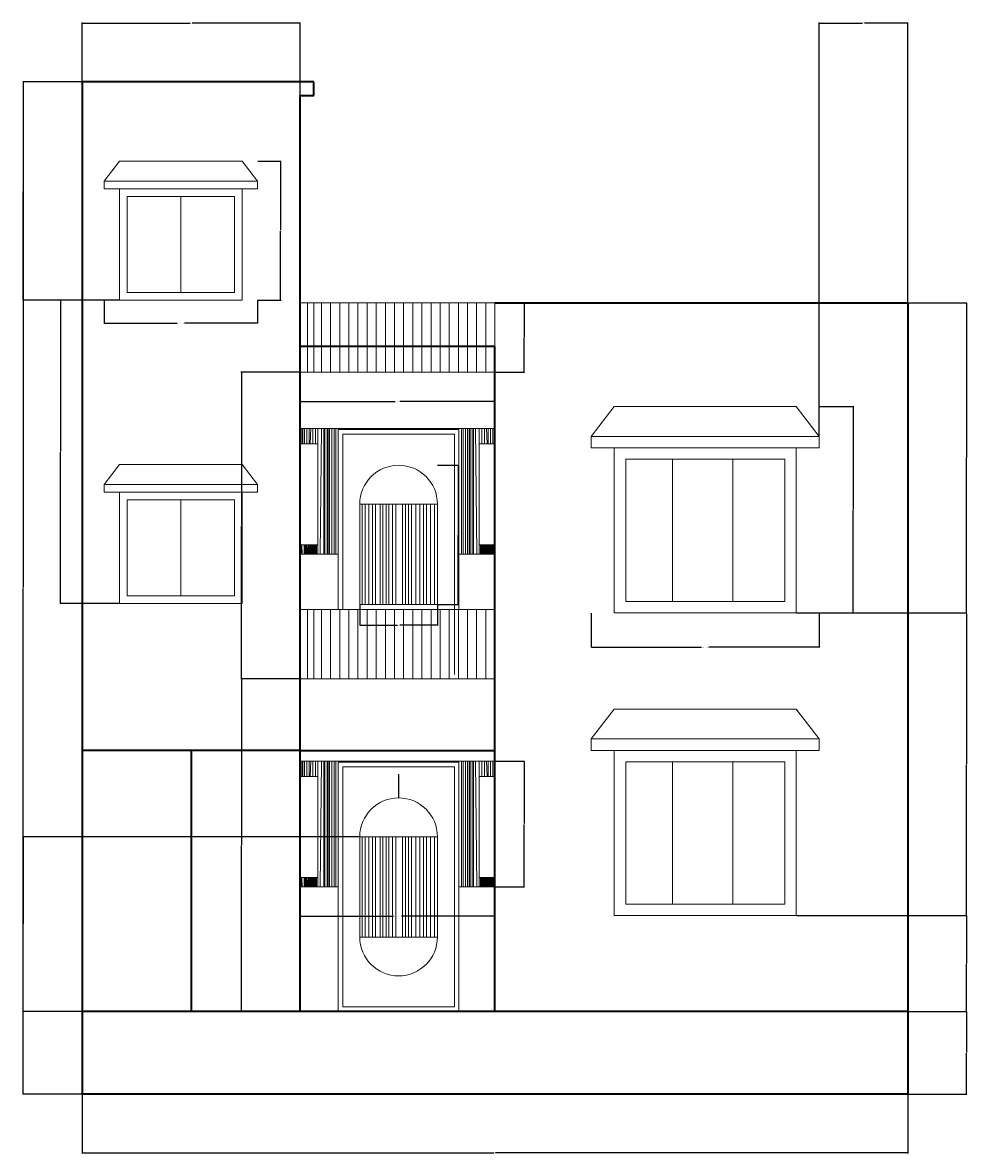
# Model space of a CAD drawing. Units: inches. Extents: x -29 to 834, y -635 to 572.
# Tile 3 of 4: x -21 to 391, y 79 to 572. Entities that reach past the tile are written whole.
import ezdxf

# ---------------------------------------------------------------- set-up
doc = ezdxf.new("R2010")
doc.units = ezdxf.units.IN
doc.header["$MEASUREMENT"] = 0
for name, color, linetype, lineweight in [('A-ANNO-DIMS', 2, 'Continuous', 18), ('A-DOOR', 3, 'Continuous', 18), ('A-ELEV', 7, 'Continuous', 35), ('A-ELEV-TRIM', 7, 'Continuous', 13), ('A-FLOR-HRAL', 3, 'Continuous', 18), ('A-GLAZ', 4, 'Continuous', 18)]:
    doc.layers.add(name, color=color, linetype=linetype, lineweight=lineweight)
doc.styles.get("Standard").update_dxf_attribs({"font": 'arial.ttf'})
doc.dimstyles.get("Standard").update_dxf_attribs({"dimtxt": 0.18, "dimasz": 0.18, "dimexe": 0.18, "dimexo": 0.0625, "dimgap": 0.09, "dimtad": 0, "dimtih": 1, "dimtoh": 1, "dimdec": 4, "dimzin": 0, "dimdsep": 46, "dimtxsty": 'Standard', "dimcen": 0.09, "dimadec": 0, "dimazin": 0, "dimtfac": 1, "dimtdec": 4, "dimtofl": 0, "dimtmove": 0, "dimatfit": 3, "dimfxl": 1, "dimtolj": 1, "dimtzin": 0, "dimarcsym": 0})

# ---------------------------------------------------------------- blocks, each defined once
blk = doc.blocks.new('WIN-HOODED-THREE-LIGHT-ELEV')
for p, q in [((10, 90.01), (0, 77.01)), ((10, 90.01), (89.35, 90.01)), ((89.35, 90.01), (99.35, 77.01)), ((0, 72.01), (0, 77.01)), ((0, 77.01), (89.35, 77.01)), ((89.35, 77.01), (99.35, 77.01)), ((99.35, 77.01), (99.35, 72.01)), ((5, 72.01), (0, 72.01)), ((10, 72.01), (5, 72.01)), ((10, 72.01), (89.35, 72.01)), ((10, 0), (10, 72.01)), ((99.35, 72.01), (89.35, 72.01)), ((89.35, 72.01), (89.35, 0)), ((35.44, 67.01), (35.44, 5)), ((61.73, 67.01), (61.73, 5)), ((89.35, 0), (10, 0))]:
    blk.add_line(p, q)
blk.add_lwpolyline([(15, 67.01), (84.35, 67.01), (84.35, 5), (15, 5)], close=True)
blk = doc.blocks.new('WIN-HOODED-TWO-LIGHT-ELEV')
for p, q in [((6.74, 60.66), (0, 51.9)), ((6.74, 60.66), (60.21, 60.66)), ((60.21, 60.66), (66.95, 51.9)), ((0, 48.53), (0, 51.9)), ((0, 51.9), (60.21, 51.9)), ((60.21, 51.9), (66.95, 51.9)), ((66.95, 51.9), (66.95, 48.53)), ((3.37, 48.53), (0, 48.53)), ((6.74, 48.53), (3.37, 48.53)), ((6.74, 48.53), (60.21, 48.53)), ((6.74, 0), (6.74, 48.53)), ((33.48, 45.16), (33.48, 3.37)), ((60.21, 48.53), (60.21, 0)), ((66.95, 48.53), (60.21, 48.53)), ((60.21, 0), (6.74, 0))]:
    blk.add_line(p, q)
blk.add_lwpolyline([(10.11, 45.16), (56.84, 45.16), (56.84, 3.37), (10.11, 3.37)], close=True)
blk = doc.blocks.new('ENTRY-SURROUND-ELEV')
for p, q in [((0, 54.81), (84.92, 54.81)), ((0.68, 54.81), (0.68, 48.11)), ((1.2, 54.81), (1.2, 48.11)), ((1.89, 54.81), (1.89, 48.11)), ((2.84, 54.81), (2.84, 48.11)), ((3.85, 54.81), (3.85, 48.11)), ((4.6, 54.81), (4.32, 48.11)), ((5.48, 54.81), (5.48, 48.11)), ((6.62, 54.81), (6.62, 48.11)), ((7.72, 0), (7.72, 54.81)), ((9.33, 54.81), (8.76, 0)), ((10.29, 0), (10.29, 54.81)), ((10.8, 54.81), (10.8, 0)), ((11.71, 0), (11.71, 54.81)), ((12.22, 54.81), (12.22, 0)), ((12.82, 0), (12.82, 54.81)), ((13.77, 54.81), (13.77, 0)), ((14.77, 0), (14.77, 54.81)), ((15.56, 54.81), (15.56, 0)), ((70.28, 54.81), (70.28, 0)), ((71.07, 0), (71.07, 54.81)), ((72.06, 54.81), (72.06, 0)), ((73.01, 0), (73.01, 54.81)), ((73.62, 54.81), (73.62, 0)), ((74.12, 0), (74.12, 54.81)), ((75.03, 54.81), (75.03, 0)), ((75.55, 0), (75.55, 54.81)), ((75.55, 54.81), (76.51, 54.81)), ((76.51, 54.81), (77.08, 0)), ((78.12, 0), (78.12, 54.81)), ((79.22, 54.81), (79.22, 48.11)), ((80.35, 54.81), (80.35, 48.11)), ((81.24, 54.81), (81.52, 48.11)), ((81.99, 54.81), (81.99, 48.11)), ((83, 54.81), (83, 48.11)), ((83.94, 54.81), (83.94, 48.11)), ((7.72, 48.11), (0, 48.11)), ((78.12, 48.11), (84.92, 48.11)), ((7.72, 4.11), (0, 4.11)), ((16.61, 0), (0, 0)), ((0.48, 4.11), (0.48, 0)), ((0.79, 4.11), (0.92, 0)), ((16.61, 0), (0.92, 0)), ((1.76, 4.11), (1.76, 0)), ((2.13, 4.11), (2.13, 0)), ((2.63, 4.11), (2.63, 0)), ((2.79, 4.11), (3.05, 0)), ((3.29, 4.11), (3.29, 0)), ((3.58, 4.11), (3.58, 0.18)), ((4, 4.11), (4, 0)), ((4.32, 4.11), (4.32, 0)), ((4.8, 4.11), (4.8, 0)), ((5.11, 4.11), (5.11, 0)), ((5.48, 4.11), (5.48, 0)), ((5.89, 4.11), (5.89, 0)), ((6.22, 4.11), (6.22, 0)), ((6.47, 4.11), (6.47, 0)), ((7.19, 0), (6.86, 4.11)), ((6.86, 4.11), (6.86, 0)), ((7.19, 4.11), (7.19, 0)), ((69.23, 0), (84.92, 0)), ((78.12, 4.11), (84.92, 4.11)), ((78.65, 4.11), (78.65, 0)), ((78.65, 0), (78.98, 4.11)), ((78.98, 4.11), (78.98, 0)), ((79.36, 4.11), (79.36, 0)), ((79.62, 4.11), (79.62, 0)), ((79.94, 4.11), (79.94, 0)), ((80.36, 4.11), (80.36, 0)), ((80.73, 4.11), (80.73, 0)), ((81.04, 4.11), (81.04, 0)), ((81.52, 4.11), (81.52, 0)), ((81.84, 4.11), (81.84, 0)), ((82.26, 4.11), (82.26, 0.18)), ((82.55, 4.11), (82.55, 0)), ((83.05, 4.11), (82.79, 0)), ((83.21, 4.11), (83.21, 0)), ((83.45, 4.11), (83.45, 0)), ((83.64, 4.11), (83.64, 0)), ((83.92, 4.11), (83.92, 0)), ((84.08, 4.11), (84.08, 0)), ((84.4, 4.11), (84.4, 0)), ((84.64, 4.11), (84.64, 0.46)), ((84.64, 0.46), (84.64, 0))]:
    blk.add_line(p, q)
blk = doc.blocks.new('DOOR-ARCHED-GRILLE-ELEV')
for p, q in [((0, 21.85), (0, 43.71)), ((0, 43.71), (33.89, 43.71)), ((1.11, 43.71), (1.11, 0)), ((2.31, 43.71), (2.31, 0)), ((3.98, 43.71), (3.98, 0)), ((5.53, 43.71), (5.53, 0)), ((6.86, 43.71), (6.86, 0)), ((8.97, 43.71), (8.97, 0)), ((10.08, 43.71), (10.08, 0)), ((11.52, 43.71), (11.52, 0)), ((12.74, 43.71), (12.74, 0)), ((14.3, 43.71), (14.3, 0)), ((15.75, 43.71), (15.75, 0)), ((18.63, 43.71), (18.63, 0)), ((19.96, 43.71), (19.96, 0)), ((21.3, 43.71), (21.3, 0)), ((22.63, 43.71), (22.63, 0)), ((24.4, 43.71), (24.4, 0)), ((26.18, 43.71), (26.18, 0)), ((27.84, 43.71), (27.84, 0)), ((29.18, 43.71), (29.18, 0)), ((30.84, 43.71), (30.84, 0)), ((32.62, 43.71), (32.62, 0)), ((33.89, 21.85), (33.89, 43.71)), ((33.89, 32.78), (33.89, 30.69)), ((33.89, 30.69), (33.89, 4.05)), ((0, 21.85), (0, 0)), ((33.89, 21.85), (33.89, 0)), ((0, 0), (33.89, 0))]:
    blk.add_line(p, q)
blk.add_arc((16.94, 43.71), 16.94, 0, 180)
blk = doc.blocks.new('RAIL-PICKET-PANEL-ELEV')
for p, q in [((84.92, 30.32), (0, 30.32)), ((3.13, 30.32), (3.13, 0)), ((5.96, 30.32), (5.96, 0)), ((9.27, 30.32), (9.27, 0)), ((13.25, 30.32), (13.25, 0)), ((17.23, 30.32), (17.23, 0)), ((21.22, 30.32), (21.22, 0)), ((25.2, 30.32), (25.2, 0)), ((29.18, 30.32), (29.18, 0)), ((33.16, 30.32), (33.16, 0)), ((37.14, 30.32), (37.14, 0)), ((41.12, 30.32), (41.12, 0)), ((45.11, 30.32), (45.11, 0)), ((49.09, 30.32), (49.09, 0)), ((53.07, 30.32), (53.07, 0)), ((57.05, 30.32), (57.05, 0)), ((61.03, 30.32), (61.03, 0)), ((65.01, 30.32), (65.01, 0)), ((69, 30.32), (69, 0)), ((72.98, 30.32), (72.98, 0)), ((76.96, 30.32), (76.96, 0)), ((80.94, 30.32), (80.94, 0)), ((84.92, 30.32), (84.92, 0)), ((84.92, 0), (0, 0))]:
    blk.add_line(p, q)
blk = doc.blocks.new('*D45')
at = {"layer": 'A-ANNO-DIMS', "color": 0, "lineweight": -2, "transparency": 16777216}
for p, q in [((227.04, 314.27), (227.04, 299.25)), ((326.38, 314.27), (326.38, 299.25)), ((227.22, 299.43), (275.08, 299.43)), ((326.2, 299.43), (278.34, 299.43))]:
    blk.add_line(p, q, dxfattribs=at)
at = {"layer": 'A-ANNO-DIMS', "color": 0, "transparency": 16777216}
for points in [[(227.22, 299.46), (227.22, 299.4), (227.04, 299.43)], [(326.2, 299.46), (326.2, 299.4), (326.38, 299.43)]]:
    blk.add_solid(points, dxfattribs=at)
at = {"layer": 'DEFPOINTS', "color": 0, "transparency": 16777216}
for p in [(227.04, 314.33), (326.38, 314.33), (326.38, 299.43)]:
    blk.add_point(p, dxfattribs=at)
at = {"layer": 'A-ANNO-DIMS', "color": 0, "transparency": 16777216, "insert": (276.71, 299.43), "char_height": 0.18, "attachment_point": 5}
blk.add_mtext('\\A1;3-LIGHT WINDOW 99 TYP.', dxfattribs=at)
blk = doc.blocks.new('*D46')
at = {"layer": 'A-ANNO-DIMS', "color": 0, "lineweight": -2, "transparency": 16777216}
for p, q in [((326.45, 404.34), (341.47, 404.34)), ((341.29, 404.16), (341.29, 359.52)), ((341.29, 314.51), (341.29, 359.15)), ((326.45, 314.33), (341.47, 314.33))]:
    blk.add_line(p, q, dxfattribs=at)
at = {"layer": 'A-ANNO-DIMS', "color": 0, "transparency": 16777216}
for points in [[(341.26, 404.16), (341.32, 404.16), (341.29, 404.34)], [(341.26, 314.51), (341.32, 314.51), (341.29, 314.33)]]:
    blk.add_solid(points, dxfattribs=at)
at = {"layer": 'DEFPOINTS', "color": 0, "transparency": 16777216}
for p in [(326.38, 404.34), (341.29, 404.34), (326.38, 314.33)]:
    blk.add_point(p, dxfattribs=at)
at = {"layer": 'A-ANNO-DIMS', "color": 0, "transparency": 16777216, "insert": (341.29, 359.33), "char_height": 0.18, "attachment_point": 5}
blk.add_mtext('\\A1;90 TYP.', dxfattribs=at)
blk = doc.blocks.new('*D47')
at = {"layer": 'A-ANNO-DIMS', "color": 0, "lineweight": -2, "transparency": 16777216}
for p, q in [((14.55, 450.67), (14.55, 440.51)), ((81.5, 450.67), (81.5, 440.51)), ((14.73, 440.69), (46.39, 440.69)), ((81.32, 440.69), (49.66, 440.69))]:
    blk.add_line(p, q, dxfattribs=at)
at = {"layer": 'A-ANNO-DIMS', "color": 0, "transparency": 16777216}
for points in [[(14.73, 440.72), (14.73, 440.66), (14.55, 440.69)], [(81.32, 440.72), (81.32, 440.66), (81.5, 440.69)]]:
    blk.add_solid(points, dxfattribs=at)
at = {"layer": 'DEFPOINTS', "color": 0, "transparency": 16777216}
for p in [(14.55, 450.73), (81.5, 450.73), (81.5, 440.69)]:
    blk.add_point(p, dxfattribs=at)
at = {"layer": 'A-ANNO-DIMS', "color": 0, "transparency": 16777216, "insert": (48.03, 440.69), "char_height": 0.18, "attachment_point": 5}
blk.add_mtext('\\A1;2-LIGHT WINDOW 67 TYP.', dxfattribs=at)
blk = doc.blocks.new('*D48')
at = {"layer": 'A-ANNO-DIMS', "color": 0, "lineweight": -2, "transparency": 16777216}
for p, q in [((81.57, 511.39), (91.73, 511.39)), ((91.55, 511.21), (91.55, 481.25)), ((91.55, 450.91), (91.55, 480.88)), ((81.57, 450.73), (91.73, 450.73))]:
    blk.add_line(p, q, dxfattribs=at)
at = {"layer": 'A-ANNO-DIMS', "color": 0, "transparency": 16777216}
for points in [[(91.52, 511.21), (91.58, 511.21), (91.55, 511.39)], [(91.52, 450.91), (91.58, 450.91), (91.55, 450.73)]]:
    blk.add_solid(points, dxfattribs=at)
at = {"layer": 'DEFPOINTS', "color": 0, "transparency": 16777216}
for p in [(81.5, 511.39), (91.55, 511.39), (81.5, 450.73)]:
    blk.add_point(p, dxfattribs=at)
at = {"layer": 'A-ANNO-DIMS', "color": 0, "transparency": 16777216, "insert": (91.55, 481.06), "char_height": 0.18, "attachment_point": 5}
blk.add_mtext('\\A1;61 TYP.', dxfattribs=at)
blk = doc.blocks.new('*D49')
at = {"layer": 'A-ANNO-DIMS', "color": 0, "lineweight": -2, "transparency": 16777216}
for p, q in [((100.09, 194.84), (100.09, 181.99)), ((185.01, 194.84), (185.01, 181.99)), ((100.27, 182.17), (140.8, 182.17)), ((184.83, 182.17), (144.29, 182.17))]:
    blk.add_line(p, q, dxfattribs=at)
at = {"layer": 'A-ANNO-DIMS', "color": 0, "transparency": 16777216}
for points in [[(100.27, 182.2), (100.27, 182.14), (100.09, 182.17)], [(184.83, 182.2), (184.83, 182.14), (185.01, 182.17)]]:
    blk.add_solid(points, dxfattribs=at)
at = {"layer": 'DEFPOINTS', "color": 0, "transparency": 16777216}
for p in [(100.09, 194.91), (185.01, 194.91), (185.01, 182.17)]:
    blk.add_point(p, dxfattribs=at)
at = {"layer": 'A-ANNO-DIMS', "color": 0, "transparency": 16777216, "insert": (142.55, 182.17), "char_height": 0.18, "attachment_point": 5}
blk.add_mtext('\\A1;ENTRY SURROUND 85 TYP.', dxfattribs=at)
blk = doc.blocks.new('*D50')
at = {"layer": 'A-ANNO-DIMS', "color": 0, "lineweight": -2, "transparency": 16777216}
for p, q in [((185.07, 249.71), (197.93, 249.71)), ((197.75, 249.53), (197.75, 222.49)), ((197.75, 195.09), (197.75, 222.13)), ((185.07, 194.91), (197.93, 194.91))]:
    blk.add_line(p, q, dxfattribs=at)
at = {"layer": 'A-ANNO-DIMS', "color": 0, "transparency": 16777216}
for points in [[(197.72, 249.53), (197.78, 249.53), (197.75, 249.71)], [(197.72, 195.09), (197.78, 195.09), (197.75, 194.91)]]:
    blk.add_solid(points, dxfattribs=at)
at = {"layer": 'DEFPOINTS', "color": 0, "transparency": 16777216}
for p in [(185.01, 249.71), (197.75, 249.71), (185.01, 194.91)]:
    blk.add_point(p, dxfattribs=at)
at = {"layer": 'A-ANNO-DIMS', "color": 0, "transparency": 16777216, "insert": (197.75, 222.31), "char_height": 0.18, "attachment_point": 5}
blk.add_mtext('\\A1;55 TYP.', dxfattribs=at)
blk = doc.blocks.new('*D51')
at = {"layer": 'A-ANNO-DIMS', "color": 0, "lineweight": -2, "transparency": 16777216}
for p, q in [((160.01, 378.74), (169.23, 378.74)), ((169.05, 378.56), (169.05, 348.6)), ((169.05, 318.27), (169.05, 348.23)), ((160.01, 318.09), (169.23, 318.09))]:
    blk.add_line(p, q, dxfattribs=at)
at = {"layer": 'A-ANNO-DIMS', "color": 0, "transparency": 16777216}
for points in [[(169.02, 378.56), (169.08, 378.56), (169.05, 378.74)], [(169.02, 318.27), (169.08, 318.27), (169.05, 318.09)]]:
    blk.add_solid(points, dxfattribs=at)
at = {"layer": 'DEFPOINTS', "color": 0, "transparency": 16777216}
for p in [(159.95, 378.74), (169.05, 378.74), (159.95, 318.09)]:
    blk.add_point(p, dxfattribs=at)
at = {"layer": 'A-ANNO-DIMS', "color": 0, "transparency": 16777216, "insert": (169.05, 348.41), "char_height": 0.18, "attachment_point": 5}
blk.add_mtext('\\A1;GRILLE 61 TYP.', dxfattribs=at)
blk = doc.blocks.new('*D52')
at = {"layer": 'A-ANNO-DIMS', "color": 0, "lineweight": -2, "transparency": 16777216}
for p, q in [((126.06, 318.03), (126.06, 308.81)), ((159.95, 318.03), (159.95, 308.81)), ((126.24, 308.99), (142.48, 308.99)), ((159.77, 308.99), (143.53, 308.99))]:
    blk.add_line(p, q, dxfattribs=at)
at = {"layer": 'A-ANNO-DIMS', "color": 0, "transparency": 16777216}
for points in [[(126.24, 309.02), (126.24, 308.96), (126.06, 308.99)], [(159.77, 309.02), (159.77, 308.96), (159.95, 308.99)]]:
    blk.add_solid(points, dxfattribs=at)
at = {"layer": 'DEFPOINTS', "color": 0, "transparency": 16777216}
for p in [(126.06, 318.09), (159.95, 318.09), (159.95, 308.99)]:
    blk.add_point(p, dxfattribs=at)
at = {"layer": 'A-ANNO-DIMS', "color": 0, "transparency": 16777216, "insert": (143.01, 308.99), "char_height": 0.18, "attachment_point": 5}
blk.add_mtext('\\A1;34 TYP.', dxfattribs=at)
blk = doc.blocks.new('*D53')
at = {"layer": 'A-ANNO-DIMS', "color": 0, "lineweight": -2, "transparency": 16777216}
for p, q in [((100.09, 419.23), (100.09, 406.37)), ((185.01, 419.23), (185.01, 406.37)), ((100.27, 406.55), (141.49, 406.55)), ((184.83, 406.55), (143.61, 406.55))]:
    blk.add_line(p, q, dxfattribs=at)
at = {"layer": 'A-ANNO-DIMS', "color": 0, "transparency": 16777216}
for points in [[(100.27, 406.58), (100.27, 406.52), (100.09, 406.55)], [(184.83, 406.58), (184.83, 406.52), (185.01, 406.55)]]:
    blk.add_solid(points, dxfattribs=at)
at = {"layer": 'DEFPOINTS', "color": 0, "transparency": 16777216}
for p in [(100.09, 419.29), (185.01, 419.29), (185.01, 406.55)]:
    blk.add_point(p, dxfattribs=at)
at = {"layer": 'A-ANNO-DIMS', "color": 0, "transparency": 16777216, "insert": (142.55, 406.55), "char_height": 0.18, "attachment_point": 5}
blk.add_mtext('\\A1;RAILING 85 TYP.', dxfattribs=at)
blk = doc.blocks.new('*D54')
at = {"layer": 'A-ANNO-DIMS', "color": 0, "lineweight": -2, "transparency": 16777216}
for p, q in [((185.07, 449.61), (197.93, 449.61)), ((197.75, 449.43), (197.75, 434.63)), ((197.75, 419.47), (197.75, 434.27)), ((185.07, 419.29), (197.93, 419.29))]:
    blk.add_line(p, q, dxfattribs=at)
at = {"layer": 'A-ANNO-DIMS', "color": 0, "transparency": 16777216}
for points in [[(197.72, 449.43), (197.78, 449.43), (197.75, 449.61)], [(197.72, 419.47), (197.78, 419.47), (197.75, 419.29)]]:
    blk.add_solid(points, dxfattribs=at)
at = {"layer": 'DEFPOINTS', "color": 0, "transparency": 16777216}
for p in [(185.01, 449.61), (197.75, 449.61), (185.01, 419.29)]:
    blk.add_point(p, dxfattribs=at)
at = {"layer": 'A-ANNO-DIMS', "color": 0, "transparency": 16777216, "insert": (197.75, 434.45), "char_height": 0.18, "attachment_point": 5}
blk.add_mtext('\\A1;30 TYP.', dxfattribs=at)
blk = doc.blocks.new('*D82')
at = {"layer": 'A-ANNO-DIMS', "color": 0, "lineweight": -2, "transparency": 16777216}
for p, q in [((5.01, 104.48), (5.01, 78.71)), ((365.01, 104.48), (365.01, 78.71)), ((5.19, 78.89), (184.72, 78.89)), ((364.83, 78.89), (185.3, 78.89))]:
    blk.add_line(p, q, dxfattribs=at)
at = {"layer": 'A-ANNO-DIMS', "color": 0, "transparency": 16777216}
for points in [[(5.19, 78.92), (5.19, 78.86), (5.01, 78.89)], [(364.83, 78.92), (364.83, 78.86), (365.01, 78.89)]]:
    blk.add_solid(points, dxfattribs=at)
at = {"layer": 'DEFPOINTS', "color": 0, "transparency": 16777216}
for p in [(5.01, 104.54), (365.01, 104.54), (365.01, 78.89)]:
    blk.add_point(p, dxfattribs=at)
at = {"layer": 'A-ANNO-DIMS', "color": 0, "transparency": 16777216, "insert": (185.01, 78.89), "char_height": 0.18, "attachment_point": 5}
blk.add_mtext('\\A1;360', dxfattribs=at)
blk = doc.blocks.new('*D83')
at = {"layer": 'A-ANNO-DIMS', "color": 0, "lineweight": -2, "transparency": 16777216}
for p, q in [((4.95, 545.91), (-20.82, 545.91)), ((-20.64, 545.73), (-20.64, 325.41)), ((-20.64, 104.72), (-20.64, 325.04)), ((4.95, 104.54), (-20.82, 104.54))]:
    blk.add_line(p, q, dxfattribs=at)
at = {"layer": 'A-ANNO-DIMS', "color": 0, "transparency": 16777216}
for points in [[(-20.67, 545.73), (-20.61, 545.73), (-20.64, 545.91)], [(-20.67, 104.72), (-20.61, 104.72), (-20.64, 104.54)]]:
    blk.add_solid(points, dxfattribs=at)
at = {"layer": 'DEFPOINTS', "color": 0, "transparency": 16777216}
for p in [(-20.64, 545.91), (5.01, 545.91), (5.01, 104.54)]:
    blk.add_point(p, dxfattribs=at)
at = {"layer": 'A-ANNO-DIMS', "color": 0, "transparency": 16777216, "insert": (-20.64, 325.23), "char_height": 0.18, "attachment_point": 5}
blk.add_mtext('\\A1;441.4', dxfattribs=at)
blk = doc.blocks.new('*D84')
at = {"layer": 'A-ANNO-DIMS', "color": 0, "lineweight": -2, "transparency": 16777216}
for p, q in [((5.01, 545.97), (5.01, 571.74)), ((5.19, 571.56), (52.15, 571.56)), ((99.91, 571.56), (52.94, 571.56)), ((100.09, 539.97), (100.09, 571.74))]:
    blk.add_line(p, q, dxfattribs=at)
at = {"layer": 'A-ANNO-DIMS', "color": 0, "transparency": 16777216}
for points in [[(5.19, 571.59), (5.19, 571.53), (5.01, 571.56)], [(99.91, 571.59), (99.91, 571.53), (100.09, 571.56)]]:
    blk.add_solid(points, dxfattribs=at)
at = {"layer": 'DEFPOINTS', "color": 0, "transparency": 16777216}
for p in [(100.09, 571.56), (5.01, 545.91), (100.09, 539.91)]:
    blk.add_point(p, dxfattribs=at)
at = {"layer": 'A-ANNO-DIMS', "color": 0, "transparency": 16777216, "insert": (52.55, 571.56), "char_height": 0.18, "attachment_point": 5}
blk.add_mtext('\\A1;95.08', dxfattribs=at)
blk = doc.blocks.new('*D85')
at = {"layer": 'A-ANNO-DIMS', "color": 0, "lineweight": -2, "transparency": 16777216}
for p, q in [((365.07, 140.54), (390.84, 140.54)), ((390.66, 140.36), (390.66, 122.72)), ((390.66, 104.72), (390.66, 122.36)), ((365.07, 104.54), (390.84, 104.54))]:
    blk.add_line(p, q, dxfattribs=at)
at = {"layer": 'A-ANNO-DIMS', "color": 0, "transparency": 16777216}
for points in [[(390.63, 140.36), (390.69, 140.36), (390.66, 140.54)], [(390.63, 104.72), (390.69, 104.72), (390.66, 104.54)]]:
    blk.add_solid(points, dxfattribs=at)
at = {"layer": 'DEFPOINTS', "color": 0, "transparency": 16777216}
for p in [(365.01, 140.54), (390.66, 140.54), (365.01, 104.54)]:
    blk.add_point(p, dxfattribs=at)
at = {"layer": 'A-ANNO-DIMS', "color": 0, "transparency": 16777216, "insert": (390.66, 122.54), "char_height": 0.18, "attachment_point": 5}
blk.add_mtext('\\A1;36', dxfattribs=at)
blk = doc.blocks.new('*D86')
at = {"layer": 'A-ANNO-DIMS', "color": 0, "lineweight": -2, "transparency": 16777216}
for p, q in [((126, 216.76), (-20.82, 216.76)), ((-20.64, 216.58), (-20.64, 178.83)), ((-20.64, 140.72), (-20.64, 178.47)), ((116.63, 140.54), (-20.82, 140.54))]:
    blk.add_line(p, q, dxfattribs=at)
at = {"layer": 'A-ANNO-DIMS', "color": 0, "transparency": 16777216}
for points in [[(-20.67, 216.58), (-20.61, 216.58), (-20.64, 216.76)], [(-20.67, 140.72), (-20.61, 140.72), (-20.64, 140.54)]]:
    blk.add_solid(points, dxfattribs=at)
at = {"layer": 'DEFPOINTS', "color": 0, "transparency": 16777216}
for p in [(-20.64, 216.76), (126.06, 216.76), (116.7, 140.54)]:
    blk.add_point(p, dxfattribs=at)
at = {"layer": 'A-ANNO-DIMS', "color": 0, "transparency": 16777216, "insert": (-20.64, 178.65), "char_height": 0.18, "attachment_point": 5}
blk.add_mtext('\\A1;76.22', dxfattribs=at)
blk = doc.blocks.new('*D87')
at = {"layer": 'A-ANNO-DIMS', "color": 0, "lineweight": -2, "transparency": 16777216}
for p, q in [((326.38, 391.4), (326.38, 571.74)), ((326.56, 571.56), (345.23, 571.56)), ((364.83, 571.56), (346.16, 571.56)), ((365.01, 449.67), (365.01, 571.74))]:
    blk.add_line(p, q, dxfattribs=at)
at = {"layer": 'A-ANNO-DIMS', "color": 0, "transparency": 16777216}
for points in [[(326.56, 571.59), (326.56, 571.53), (326.38, 571.56)], [(364.83, 571.59), (364.83, 571.53), (365.01, 571.56)]]:
    blk.add_solid(points, dxfattribs=at)
at = {"layer": 'DEFPOINTS', "color": 0, "transparency": 16777216}
for p in [(365.01, 571.56), (365.01, 449.61), (326.38, 391.34)]:
    blk.add_point(p, dxfattribs=at)
at = {"layer": 'A-ANNO-DIMS', "color": 0, "transparency": 16777216, "insert": (345.7, 571.56), "char_height": 0.18, "attachment_point": 5}
blk.add_mtext('\\A1;38.626', dxfattribs=at)
blk = doc.blocks.new('*D88')
at = {"layer": 'A-ANNO-DIMS', "color": 0, "lineweight": -2, "transparency": 16777216}
for p, q in [((316.45, 182.44), (390.84, 182.44)), ((390.66, 182.26), (390.66, 161.67)), ((390.66, 140.72), (390.66, 161.31)), ((365.07, 140.54), (390.84, 140.54))]:
    blk.add_line(p, q, dxfattribs=at)
at = {"layer": 'A-ANNO-DIMS', "color": 0, "transparency": 16777216}
for points in [[(390.63, 182.26), (390.69, 182.26), (390.66, 182.44)], [(390.63, 140.72), (390.69, 140.72), (390.66, 140.54)]]:
    blk.add_solid(points, dxfattribs=at)
at = {"layer": 'DEFPOINTS', "color": 0, "transparency": 16777216}
for p in [(316.38, 182.44), (365.01, 140.54), (390.66, 140.54)]:
    blk.add_point(p, dxfattribs=at)
at = {"layer": 'A-ANNO-DIMS', "color": 0, "transparency": 16777216, "insert": (390.66, 161.49), "char_height": 0.18, "attachment_point": 5}
blk.add_mtext('\\A1;41.89', dxfattribs=at)
blk = doc.blocks.new('*D89')
at = {"layer": 'A-ANNO-DIMS', "color": 0, "lineweight": -2, "transparency": 16777216}
for p, q in [((316.45, 314.33), (390.84, 314.33)), ((390.66, 314.15), (390.66, 248.56)), ((390.66, 182.62), (390.66, 248.2)), ((316.45, 182.44), (390.84, 182.44))]:
    blk.add_line(p, q, dxfattribs=at)
at = {"layer": 'A-ANNO-DIMS', "color": 0, "transparency": 16777216}
for points in [[(390.63, 314.15), (390.69, 314.15), (390.66, 314.33)], [(390.63, 182.62), (390.69, 182.62), (390.66, 182.44)]]:
    blk.add_solid(points, dxfattribs=at)
at = {"layer": 'DEFPOINTS', "color": 0, "transparency": 16777216}
for p in [(316.38, 314.33), (390.66, 314.33), (316.38, 182.44)]:
    blk.add_point(p, dxfattribs=at)
at = {"layer": 'A-ANNO-DIMS', "color": 0, "transparency": 16777216, "insert": (390.66, 248.38), "char_height": 0.18, "attachment_point": 5}
blk.add_mtext('\\A1;131.9', dxfattribs=at)
blk = doc.blocks.new('*D90')
at = {"layer": 'A-ANNO-DIMS', "color": 0, "lineweight": -2, "transparency": 16777216}
for p, q in [((365.07, 449.61), (390.84, 449.61)), ((390.66, 449.43), (390.66, 382.15)), ((390.66, 314.51), (390.66, 381.79)), ((316.45, 314.33), (390.84, 314.33))]:
    blk.add_line(p, q, dxfattribs=at)
at = {"layer": 'A-ANNO-DIMS', "color": 0, "transparency": 16777216}
for points in [[(390.63, 449.43), (390.69, 449.43), (390.66, 449.61)], [(390.63, 314.51), (390.69, 314.51), (390.66, 314.33)]]:
    blk.add_solid(points, dxfattribs=at)
at = {"layer": 'DEFPOINTS', "color": 0, "transparency": 16777216}
for p in [(365.01, 449.61), (390.66, 449.61), (316.38, 314.33)]:
    blk.add_point(p, dxfattribs=at)
at = {"layer": 'A-ANNO-DIMS', "color": 0, "transparency": 16777216, "insert": (390.66, 381.97), "char_height": 0.18, "attachment_point": 5}
blk.add_mtext('\\A1;135.28', dxfattribs=at)
blk = doc.blocks.new('*D91')
at = {"layer": 'A-ANNO-DIMS', "color": 0, "lineweight": -2, "transparency": 16777216}
for p, q in [((100.02, 285.58), (74.26, 285.58)), ((74.44, 285.4), (74.44, 213.24)), ((74.44, 140.72), (74.44, 212.88)), ((100.02, 140.54), (74.26, 140.54))]:
    blk.add_line(p, q, dxfattribs=at)
at = {"layer": 'A-ANNO-DIMS', "color": 0, "transparency": 16777216}
for points in [[(74.41, 285.4), (74.47, 285.4), (74.44, 285.58)], [(74.41, 140.72), (74.47, 140.72), (74.44, 140.54)]]:
    blk.add_solid(points, dxfattribs=at)
at = {"layer": 'DEFPOINTS', "color": 0, "transparency": 16777216}
for p in [(74.44, 285.58), (100.09, 285.58), (100.09, 140.54)]:
    blk.add_point(p, dxfattribs=at)
at = {"layer": 'A-ANNO-DIMS', "color": 0, "transparency": 16777216, "insert": (74.44, 213.06), "char_height": 0.18, "attachment_point": 5}
blk.add_mtext('\\A1;145.04', dxfattribs=at)
blk = doc.blocks.new('*D92')
at = {"layer": 'A-ANNO-DIMS', "color": 0, "lineweight": -2, "transparency": 16777216}
for p, q in [((100.02, 419.29), (74.26, 419.29)), ((74.44, 419.11), (74.44, 352.61)), ((74.44, 285.76), (74.44, 352.25)), ((100.02, 285.58), (74.26, 285.58))]:
    blk.add_line(p, q, dxfattribs=at)
at = {"layer": 'A-ANNO-DIMS', "color": 0, "transparency": 16777216}
for points in [[(74.41, 419.11), (74.47, 419.11), (74.44, 419.29)], [(74.41, 285.76), (74.47, 285.76), (74.44, 285.58)]]:
    blk.add_solid(points, dxfattribs=at)
at = {"layer": 'DEFPOINTS', "color": 0, "transparency": 16777216}
for p in [(74.44, 419.29), (100.09, 419.29), (100.09, 285.58)]:
    blk.add_point(p, dxfattribs=at)
at = {"layer": 'A-ANNO-DIMS', "color": 0, "transparency": 16777216, "insert": (74.44, 352.43), "char_height": 0.18, "attachment_point": 5}
blk.add_mtext('\\A1;133.7', dxfattribs=at)
blk = doc.blocks.new('*D93')
at = {"layer": 'A-ANNO-DIMS', "color": 0, "lineweight": -2, "transparency": 16777216}
for p, q in [((21.23, 450.73), (-4.54, 450.73)), ((-4.36, 450.55), (-4.36, 384.78)), ((-4.36, 318.63), (-4.36, 384.41)), ((21.23, 318.45), (-4.54, 318.45))]:
    blk.add_line(p, q, dxfattribs=at)
at = {"layer": 'A-ANNO-DIMS', "color": 0, "transparency": 16777216}
for points in [[(-4.39, 450.55), (-4.33, 450.55), (-4.36, 450.73)], [(-4.39, 318.63), (-4.33, 318.63), (-4.36, 318.45)]]:
    blk.add_solid(points, dxfattribs=at)
at = {"layer": 'DEFPOINTS', "color": 0, "transparency": 16777216}
for p in [(-4.36, 450.73), (21.29, 450.73), (21.29, 318.45)]:
    blk.add_point(p, dxfattribs=at)
at = {"layer": 'A-ANNO-DIMS', "color": 0, "transparency": 16777216, "insert": (-4.36, 384.59), "char_height": 0.18, "attachment_point": 5}
blk.add_mtext('\\A1;132.28', dxfattribs=at)
blk = doc.blocks.new('*D94')
at = {"layer": 'A-ANNO-DIMS', "color": 0, "lineweight": -2, "transparency": 16777216}
for p, q in [((4.95, 545.91), (-20.82, 545.91)), ((-20.64, 545.73), (-20.64, 498.5)), ((-20.64, 450.91), (-20.64, 498.14)), ((21.23, 450.73), (-20.82, 450.73))]:
    blk.add_line(p, q, dxfattribs=at)
at = {"layer": 'A-ANNO-DIMS', "color": 0, "transparency": 16777216}
for points in [[(-20.67, 545.73), (-20.61, 545.73), (-20.64, 545.91)], [(-20.67, 450.91), (-20.61, 450.91), (-20.64, 450.73)]]:
    blk.add_solid(points, dxfattribs=at)
at = {"layer": 'DEFPOINTS', "color": 0, "transparency": 16777216}
for p in [(-20.64, 545.91), (5.01, 545.91), (21.29, 450.73)]:
    blk.add_point(p, dxfattribs=at)
at = {"layer": 'A-ANNO-DIMS', "color": 0, "transparency": 16777216, "insert": (-20.64, 498.32), "char_height": 0.18, "attachment_point": 5}
blk.add_mtext('\\A1;95.17', dxfattribs=at)
blk = doc.blocks.new('*D109')
at = {"layer": 'A-ANNO-DIMS', "color": 0, "lineweight": -2, "transparency": 16777216}
for p, q in [((142.83, 243.87), (143.01, 243.87)), ((143.01, 243.87), (143.01, 233.89)), ((142.92, 216.76), (143.1, 216.76)), ((143.01, 216.67), (143.01, 216.85))]:
    blk.add_line(p, q, dxfattribs=at)
at = {"layer": 'A-ANNO-DIMS', "color": 0, "transparency": 16777216}
blk.add_solid([(143.04, 233.89), (142.98, 233.89), (143.01, 233.71)], dxfattribs=at)
at = {"layer": 'DEFPOINTS', "color": 0, "transparency": 16777216}
for p in [(143.01, 233.71), (143.01, 216.76)]:
    blk.add_point(p, dxfattribs=at)
at = {"layer": 'A-ANNO-DIMS', "color": 0, "transparency": 16777216, "insert": (142.08, 243.87), "char_height": 0.18, "attachment_point": 5}
blk.add_mtext('\\A1;3X R16.945', dxfattribs=at)

msp = doc.modelspace()

# ---------------------------------------------------------------- linework, layer by layer
at = {"layer": 'A-DOOR'}
for p, q in [((118.6975, 392.307), (167.3149, 392.307)), ((118.6975, 315.8993), (118.6975, 392.307)), ((167.3149, 392.307), (167.3149, 287.5766))]:
    msp.add_line(p, q, dxfattribs=at)
msp.add_lwpolyline([(116.6975, 315.8993), (116.6975, 394.307), (169.3149, 394.307), (169.3149, 315.8993)], dxfattribs=at)
for points in [[(116.6975, 249.272), (169.3149, 249.272), (169.3149, 140.5416), (116.6975, 140.5416)], [(118.6975, 247.272), (167.3149, 247.272), (167.3149, 142.5416), (118.6975, 142.5416)]]:
    msp.add_lwpolyline(points, close=True, dxfattribs=at)
msp.add_arc((143.0062, 173.053), 16.9446, 180, 0, dxfattribs=at)
at = {"layer": 'A-ELEV'}
for p, q in [((106.087, 545.9086), (5.0102, 545.9086)), ((5.0102, 545.9086), (5.0102, 104.5416)), ((106.087, 539.9086), (106.087, 545.9086)), ((100.087, 430.6116), (100.087, 539.9086)), ((100.087, 539.9086), (100.087, 539.9086)), ((100.087, 539.9086), (106.087, 539.9086)), ((185.0102, 449.6103), (365.0102, 449.6103)), ((365.0102, 449.6103), (365.0102, 104.5416)), ((100.087, 140.5416), (100.087, 430.6116)), ((100.087, 430.6116), (185.0102, 430.6116)), ((185.0102, 140.5416), (185.0102, 430.6116)), ((100.087, 254.4461), (5.0102, 254.4461)), ((52.5486, 254.4461), (52.5486, 140.5416)), ((100.087, 254.4461), (185.0102, 254.4461)), ((365.0102, 140.5416), (5.0102, 140.5416)), ((365.0102, 104.5416), (5.0102, 104.5416))]:
    msp.add_line(p, q, dxfattribs=at)
at = {"layer": 'A-ELEV-TRIM'}
for points in [[(169.3149, 419.2876), (116.6975, 419.2876)], [(169.3149, 285.5766), (116.6975, 285.5766)]]:
    msp.add_lwpolyline(points, dxfattribs=at)

# ---------------------------------------------------------------- block references
at = {"layer": 'A-DOOR'}
for p in [(126.0616, 318.088), (126.0616, 173.053)]:
    msp.add_blockref('DOOR-ARCHED-GRILLE-ELEV', p, dxfattribs=at)
at = {"layer": 'A-ELEV-TRIM'}
for p in [(100.087, 339.9418), (100.087, 194.9068)]:
    msp.add_blockref('ENTRY-SURROUND-ELEV', p, dxfattribs=at)
at = {"layer": 'A-FLOR-HRAL'}
for p in [(100.087, 419.2876), (100.087, 285.5766)]:
    msp.add_blockref('RAIL-PICKET-PANEL-ELEV', p, dxfattribs=at)
at = {"layer": 'A-GLAZ'}
for name, p in [('WIN-HOODED-TWO-LIGHT-ELEV', (14.5529, 450.7344)), ('WIN-HOODED-THREE-LIGHT-ELEV', (227.0372, 314.3291)), ('WIN-HOODED-TWO-LIGHT-ELEV', (14.5529, 318.4523)), ('WIN-HOODED-THREE-LIGHT-ELEV', (227.0372, 182.4355))]:
    msp.add_blockref(name, p, dxfattribs=at)

# ---------------------------------------------------------------- dimensions: what is measured, and where the dimension line sits
at = {"layer": 'A-ANNO-DIMS'}
for base, p1, p2, override, picture, middle in [((100.087, 571.5586), (5.0102, 545.9086), (100.087, 539.9086), {"dimdec": 2, "dimlfac": 1, "dimrnd": 0, "dimzin": 0, "dimdsep": 46, "dimlunit": 2}, '*D84', (52.5486, 571.5586)), ((365.0102, 571.5586), (326.3844, 391.3397), (365.0102, 449.6103), {"dimdec": 3, "dimlfac": 1, "dimrnd": 0, "dimzin": 0, "dimdsep": 46, "dimlunit": 2}, '*D87', (345.6973, 571.5586)), ((365.0102, 78.8916), (5.0102, 104.5416), (365.0102, 104.5416), {"dimdec": 0, "dimlfac": 1, "dimrnd": 0, "dimzin": 0, "dimdsep": 46, "dimlunit": 2}, '*D82', (185.0102, 78.8916))]:
    dim = msp.add_linear_dim(base=base, p1=p1, p2=p2, dimstyle='Standard', override=override, dxfattribs=at)
    dim.commit()
    dim.dimension.update_dxf_attribs({"geometry": picture, "text_midpoint": middle})
for base, p1, p2, override, picture, middle in [((-20.6398, 545.9086), (5.0102, 104.5416), (5.0102, 545.9086), {"dimdec": 1, "dimlfac": 1, "dimrnd": 0, "dimzin": 0, "dimdsep": 46, "dimlunit": 2}, '*D83', (-20.6398, 325.2251)), ((-20.6398, 545.9086), (21.2919, 450.7344), (5.0102, 545.9086), {"dimdec": 2, "dimlfac": 1, "dimrnd": 0, "dimzin": 0, "dimdsep": 46, "dimlunit": 2}, '*D94', (-20.6398, 498.3215)), ((-4.3581, 450.7344), (21.2919, 318.4523), (21.2919, 450.7344), {"dimdec": 2, "dimlfac": 1, "dimrnd": 0, "dimzin": 0, "dimdsep": 46, "dimlunit": 2}, '*D93', (-4.3581, 384.5933)), ((390.6602, 449.6103), (316.3844, 314.3291), (365.0102, 449.6103), {"dimdec": 2, "dimlfac": 1, "dimrnd": 0, "dimzin": 0, "dimdsep": 46, "dimlunit": 2}, '*D90', (390.6602, 381.9697)), ((74.437, 419.2876), (100.087, 285.5766), (100.087, 419.2876), {"dimdec": 1, "dimlfac": 1, "dimrnd": 0, "dimzin": 0, "dimdsep": 46, "dimlunit": 2}, '*D92', (74.437, 352.4321)), ((390.6602, 314.3291), (316.3844, 182.4355), (316.3844, 314.3291), {"dimdec": 1, "dimlfac": 1, "dimrnd": 0, "dimzin": 0, "dimdsep": 46, "dimlunit": 2}, '*D89', (390.6602, 248.3823)), ((74.43702, 285.57661), (100.08702, 140.5416), (100.08702, 285.57661), {"dimdec": 2, "dimlfac": 1, "dimrnd": 0, "dimzin": 0, "dimdsep": 46, "dimlunit": 2}, '*D91', (74.43702, 213.0591)), ((-20.6398, 216.7606), (116.6975, 140.5416), (126.0616, 216.7606), {"dimdec": 2, "dimlfac": 1, "dimrnd": 0, "dimzin": 0, "dimdsep": 46, "dimlunit": 2}, '*D86', (-20.6398, 178.6511)), ((390.6602, 140.5416), (316.3844, 182.4355), (365.0102, 140.5416), {"dimdec": 2, "dimlfac": 1, "dimrnd": 0, "dimzin": 0, "dimdsep": 46, "dimlunit": 2}, '*D88', (390.6602, 161.4885)), ((390.6602, 140.5416), (365.0102, 104.5416), (365.0102, 140.5416), {"dimdec": 0, "dimlfac": 1, "dimrnd": 0, "dimzin": 0, "dimdsep": 46, "dimlunit": 2}, '*D85', (390.6602, 122.5416))]:
    dim = msp.add_linear_dim(base=base, p1=p1, p2=p2, angle=90, dimstyle='Standard', override=override, dxfattribs=at)
    dim.commit()
    dim.dimension.update_dxf_attribs({"geometry": picture, "text_midpoint": middle})
for base, p1, p2, text, picture, middle in [((91.5455, 511.3926), (81.503, 450.7344), (81.503, 511.3926), '<> TYP.', '*D48', (91.5455, 481.0635)), ((197.7487, 449.6103), (185.0102, 419.2876), (185.0102, 449.6103), '<> TYP.', '*D54', (197.7487, 434.4489)), ((341.2864, 404.3397), (326.3844, 314.3291), (326.3844, 404.3397), '<> TYP.', '*D46', (341.2864, 359.3344)), ((169.0486, 378.7402), (159.9508, 318.088), (159.9508, 378.7402), 'GRILLE <> TYP.', '*D51', (169.0486, 348.4141)), ((197.7487, 249.7127), (185.0102, 194.9068), (185.0102, 249.7127), '<> TYP.', '*D50', (197.7487, 222.3097))]:
    dim = msp.add_linear_dim(base=base, p1=p1, p2=p2, angle=90, text=text, dimstyle='Standard', override={"dimdec": 0, "dimlfac": 1, "dimrnd": 0, "dimzin": 0, "dimdsep": 46, "dimlunit": 2}, dxfattribs=at)
    dim.commit()
    dim.dimension.update_dxf_attribs({"geometry": picture, "text_midpoint": middle})
for base, p1, p2, text, picture, middle in [((81.503, 440.6918), (14.5529, 450.7344), (81.503, 450.7344), '2-LIGHT WINDOW <> TYP.', '*D47', (48.028, 440.6918)), ((185.0102, 406.5491), (100.087, 419.2876), (185.0102, 419.2876), 'RAILING <> TYP.', '*D53', (142.5486, 406.5491)), ((159.9508, 308.9902), (126.0616, 318.088), (159.9508, 318.088), '<> TYP.', '*D52', (143.0062, 308.9902)), ((326.3844, 299.427), (227.0372, 314.3291), (326.3844, 314.3291), '3-LIGHT WINDOW <> TYP.', '*D45', (276.7108, 299.427)), ((185.0102, 182.1683), (100.087, 194.9068), (185.0102, 194.9068), 'ENTRY SURROUND <> TYP.', '*D49', (142.5486, 182.1683))]:
    dim = msp.add_linear_dim(base=base, p1=p1, p2=p2, text=text, dimstyle='Standard', override={"dimdec": 0, "dimlfac": 1, "dimrnd": 0, "dimzin": 0, "dimdsep": 46, "dimlunit": 2}, dxfattribs=at)
    dim.commit()
    dim.dimension.update_dxf_attribs({"geometry": picture, "text_midpoint": middle})
dim = msp.add_radius_dim(center=(143.0062, 216.7606), mpoint=(143.006, 233.7052), text='3X <>', dimstyle='Standard', override={"dimdec": 3, "dimlfac": 1, "dimrnd": 0, "dimzin": 0, "dimdsep": 46, "dimlunit": 2}, dxfattribs=at)
dim.commit()
dim.dimension.update_dxf_attribs({"geometry": '*D109', "text_midpoint": (142.0821, 243.8719), "dimtype": 164})

doc.saveas('drawing.dxf')
